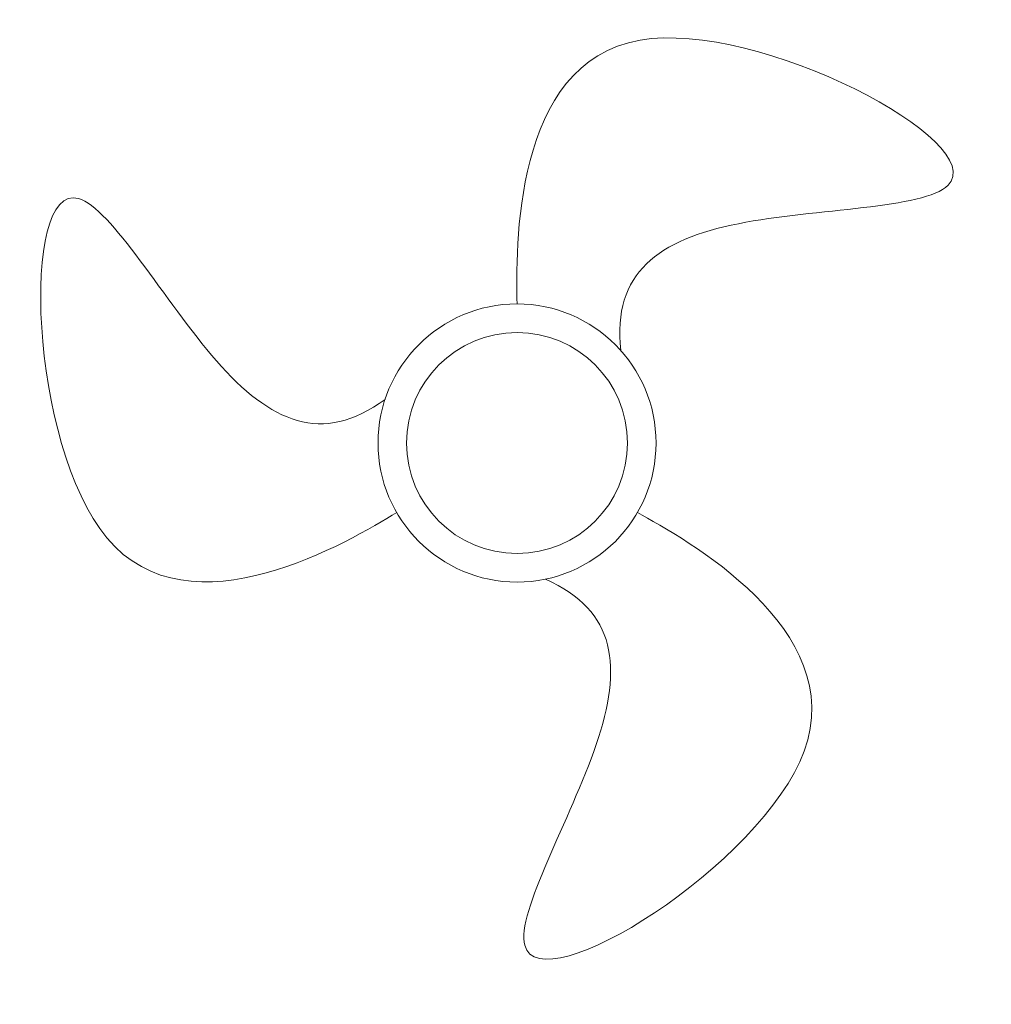
# Model space of a CAD drawing. Units: millimetres. Extents: x 3272.1 to 3302.4, y 1483.3 to 1514.
import ezdxf

# ---------------------------------------------------------------- set-up
doc = ezdxf.new("R2010")
doc.units = ezdxf.units.MM
doc.layers.add('M-CONS', color=8, linetype='Continuous', lineweight=18)

msp = doc.modelspace()

# ---------------------------------------------------------------- linework, layer by layer
at = {"layer": 'M-CONS'}
for radius in [4.34, 4.34, 4.34, 4.34, 3.45]:
    msp.add_circle((3287.599, 1500.769), radius, dxfattribs=at)
for points in [[(3287.599, 1505.109), (3287.567, 1506.755), (3287.317, 1518.111), (3306.424, 1508.034), (3293.401, 1508.112), (3290.572, 1506.084), (3290.838, 1503.658)], [(3283.841, 1498.599), (3282.432, 1497.747), (3272.721, 1491.852), (3271.895, 1513.438), (3278.339, 1502.121), (3281.51, 1500.685), (3283.478, 1502.128)], [(3291.358, 1498.599), (3292.8, 1497.804), (3302.76, 1492.342), (3284.479, 1480.834), (3291.058, 1492.073), (3290.717, 1495.537), (3288.483, 1496.519)]]:
    msp.add_open_spline(points, degree=3, knots=[0, 0, 0, 0, 3.768314, 7.258593, 9.190423, 11.198104, 11.198104, 11.198104, 11.198104], dxfattribs=at)

doc.saveas('drawing.dxf')
